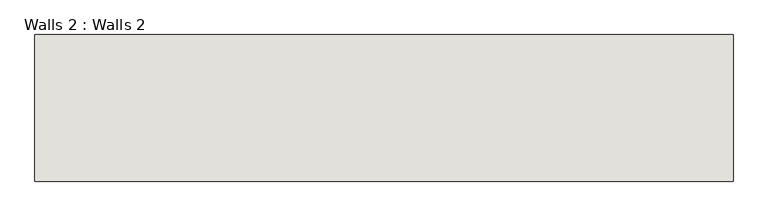
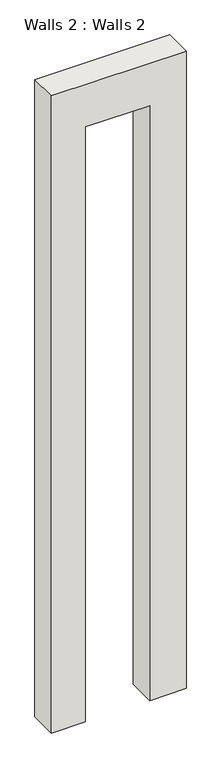
"""IFC4 building model written with IfcOpenShell, lengths in millimetres: wall geometry, Walls 2 : Walls 2."""

from ifc_helpers import new_model, si_unit, frame, origin, place, context, project, spatial, polyline, outline, extrude, source, transform, mapped, element, save


def walls_2_walls_2_8cca178c(model_context):
    return source(origin(), model_context, "Body", "SweptSolid", [
        extrude(outline(polyline([(16002.0, -6633.9371298), (16002.0, -9834.3371298), (0.0, -9834.3371298), (0.0, -9024.7121298), (14935.2, -9024.7121298), (14935.2, -7497.5371298), (0.0, -7497.5371298), (0.0, -6633.9371298), (16002.0, -6633.9371298)])), frame((0.0, 674.377413, 0.0), z_axis=(0.0, 1.0, 0.0), x_axis=(0.0, 0.0, 1.0)), (0.0, 0.0, 1.0), 673.3585688),
    ])


if __name__ == "__main__":
    model = new_model("IFC4")
    model_context = context("Model", 3, world=origin())
    ifc_project = project(units=[si_unit("LENGTHUNIT", "METRE", prefix="MILLI")], contexts=[model_context])
    site = spatial("IfcSite", under=ifc_project)
    building = spatial("IfcBuilding", under=site)
    placement = place(None, origin())
    walls_2_walls_2_shape = walls_2_walls_2_8cca178c(model_context)
    element("IfcWall", 1, ObjectType="Walls 2 : Walls 2", at=placement, inside=building, context=model_context, shape_type="MappedRepresentation", body=[
        mapped(walls_2_walls_2_shape, transform((0.0, 0.0, 0.0), x_axis=(1.0, 0.0, 0.0), y_axis=(0.0, 1.0, 0.0), z_axis=(0.0, 0.0, 1.0))),
    ])
    save(model, "model.ifc")

# Revit data of these elements
# Element 1 (IfcWall, "Walls 2 : Walls 2")
#   Materials on its faces: "Default Wall"
# Materials
#   "Default Wall": colour RGB 128 128 128, transparency 0
